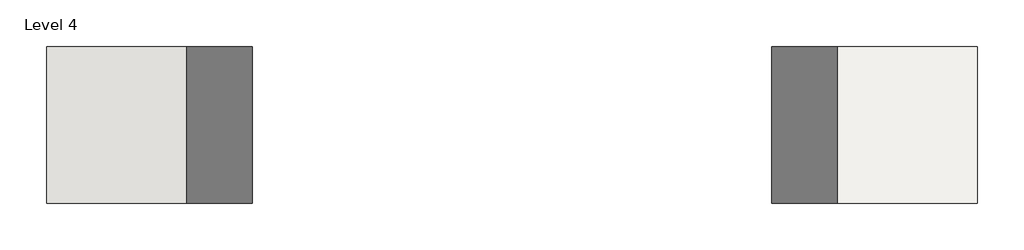
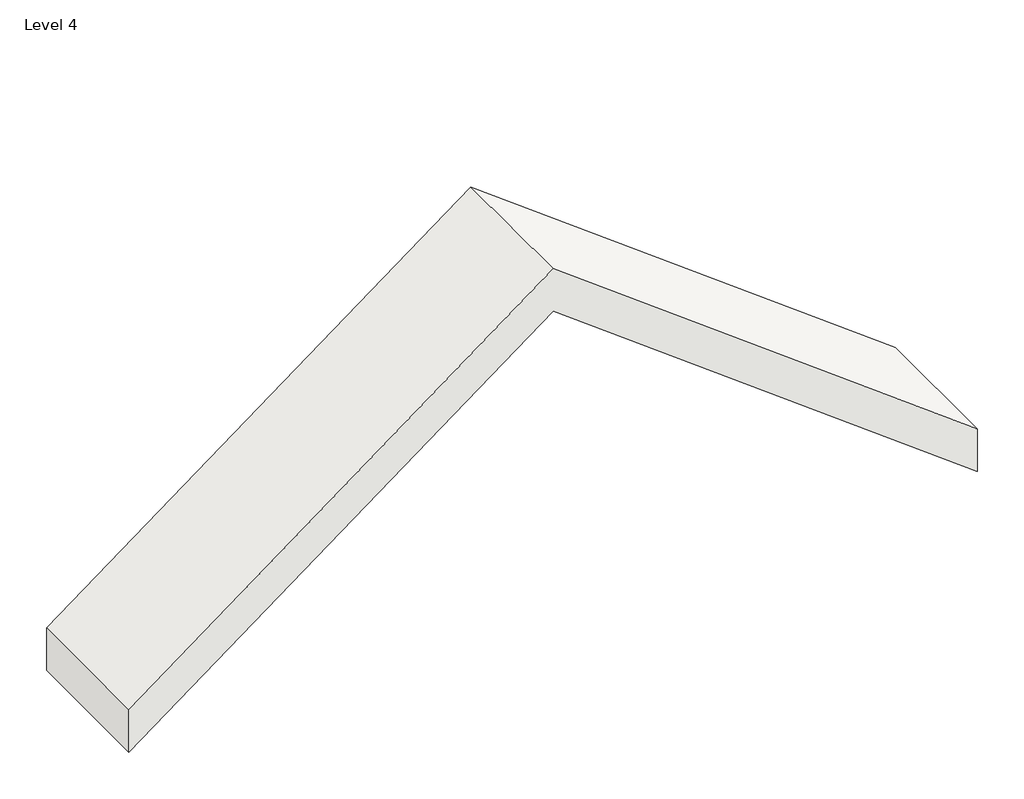
# One storey: 1 roof.
"""IFC4 building model written with IfcOpenShell, lengths in millimetres."""

from ifc_helpers import new_model, si_unit, frame, origin, place, context, project, spatial, polyline, outline, extrude, element, save

model = new_model("IFC4")

# Units and contexts
model_context = context("Model", 3, world=origin())
ifc_project = project(units=[si_unit("LENGTHUNIT", "METRE", prefix="MILLI")], contexts=[model_context])

# Site, building, storey
site = spatial("IfcSite", under=ifc_project)
building = spatial("IfcBuilding", under=site)
storey = spatial("IfcBuildingStorey", under=building, Name="Level 4", Elevation=9144.0)

# Roof
placement = place(None, origin())
element("IfcRoof", 1, ObjectType="Generic - 12\"", at=placement, inside=storey, context=model_context, shape_type="SweptSolid", body=[
    extrude(outline(polyline([(9525.0, 14466.2788287), (12242.158248, 10843.4011647), (9525.0, 7220.5235008), (9144.0, 7220.5235008), (11861.158248, 10843.4011647), (9144.0, 14466.2788287), (9525.0, 14466.2788287)])), frame((0.0, -13839.8436591, 0.0), z_axis=(0.0, 1.0, 0.0), x_axis=(0.0, 0.0, 1.0)), (0.0, 0.0, 1.0), 1219.2),
])

save(model, "model.ifc")

# Revit data of these elements
# Type "Generic - 12\""
#   Assembly Code = "B1020"
#   Layers, outside or top first: 1' - 0" no material (function 1)
# Element 1 (IfcRoof, "Generic - 12\"")
#   built-in parameter 1001705 = 40.1646 (stored number, unit not read)
#   built-in parameter 1001710 = 33615
#   Phase Created = New Construction
#   Materials on its faces: "Default Roof"
# Materials
#   "Default Roof": colour RGB 88 101 114, transparency 0, Cost = 0
